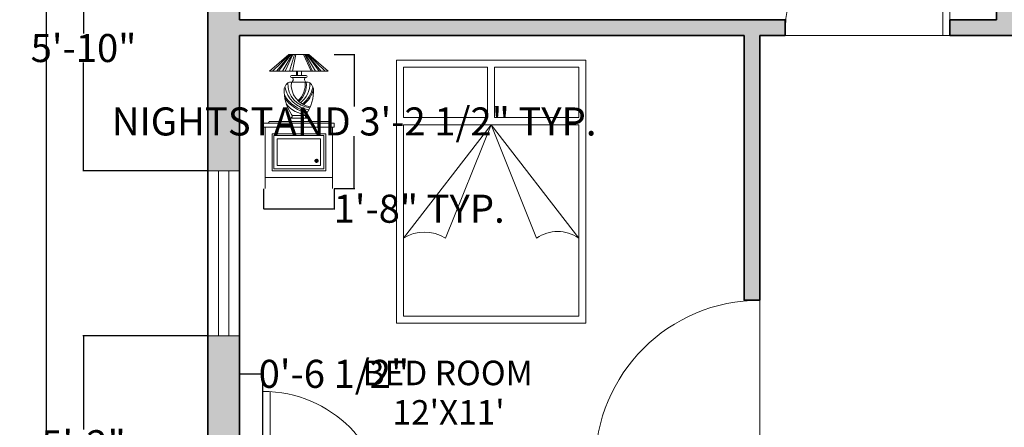
# Model space of a CAD drawing. Units: inches. Extents: x 638 to 1303, y 1 to 699.
# Tile 10 of 21: x 644 to 924, y 409 to 525. Entities that reach past the tile are written whole.
import ezdxf

# ---------------------------------------------------------------- set-up
doc = ezdxf.new("R2010")
doc.units = ezdxf.units.IN
doc.header["$MEASUREMENT"] = 0
for name, color, linetype, lineweight in [('A-ANNO-DIMS', 2, 'Continuous', 18), ('A-AREA-IDEN', 7, 'Continuous', 18), ('A-DOOR', 4, 'Continuous', 18), ('A-GLAZ', 4, 'Continuous', 18), ('A-WALL', 7, 'Continuous', 35), ('Furniture', 7, 'Continuous', 15)]:
    doc.layers.add(name, color=color, linetype=linetype, lineweight=lineweight)
doc.layers.add('A-WALL-PATT', color=143, linetype='Continuous', lineweight=13, true_color=0x7aafdf)
doc.styles.get("Standard").update_dxf_attribs({"font": 'arial.ttf'})
doc.dimstyles.get("Standard").update_dxf_attribs({"dimtxt": 8, "dimasz": 0.18, "dimexe": 0.18, "dimexo": 0.0625, "dimgap": 0.09, "dimtad": 0, "dimtih": 1, "dimtoh": 1, "dimdec": 4, "dimzin": 0, "dimdsep": 46, "dimlunit": 3, "dimtxsty": 'Standard', "dimcen": 0.09, "dimadec": 0, "dimazin": 0, "dimtfac": 1, "dimtdec": 4, "dimtofl": 0, "dimtmove": 0, "dimatfit": 3, "dimfxl": 1, "dimtolj": 1, "dimtzin": 0, "dimarcsym": 0})

# ---------------------------------------------------------------- blocks, each defined once
blk = doc.blocks.new('*D1')
at = {"layer": 'A-ANNO-DIMS', "color": 0, "lineweight": -2, "transparency": 16777216}
for p, q in [((697.18, 629.82), (650.92, 629.82)), ((651.1, 629.64), (651.1, 339.99)), ((651.1, 42), (651.1, 331.64)), ((697.18, 41.82), (650.92, 41.82))]:
    blk.add_line(p, q, dxfattribs=at)
at = {"layer": 'A-ANNO-DIMS', "color": 0, "transparency": 16777216}
for points in [[(651.07, 629.64), (651.13, 629.64), (651.1, 629.82)], [(651.07, 42), (651.13, 42), (651.1, 41.82)]]:
    blk.add_solid(points, dxfattribs=at)
at = {"layer": 'Defpoints', "color": 0, "transparency": 16777216}
for p in [(697.24, 629.82), (651.1, 41.82), (697.24, 41.82)]:
    blk.add_point(p, dxfattribs=at)
at = {"layer": 'A-ANNO-DIMS', "color": 0, "transparency": 16777216, "insert": (651.1, 335.82), "char_height": 8, "attachment_point": 5}
blk.add_mtext("\\A1;49'", dxfattribs=at)
blk = doc.blocks.new('DOOR-SWING-47')
for p, q in [((45, 0), (45, 46.96)), ((47, 0), (47, 47)), ((0, 0), (47, 0))]:
    blk.add_line(p, q)
blk.add_arc((47, 0), 47, 90, 180)
blk = doc.blocks.new('DOOR-SWING-35')
for p, q in [((33, 0), (33, 34.94)), ((35, 0), (35, 35)), ((0, 0), (35, 0))]:
    blk.add_line(p, q)
blk.add_arc((35, 0), 35, 90, 180)
blk = doc.blocks.new('WIN-47')
for p, q in [((47, 9), (0, 9)), ((0, 9), (0, 0)), ((47, 0), (47, 9)), ((0, 6), (47, 6)), ((0, 3), (47, 3)), ((0, 0), (47, 0))]:
    blk.add_line(p, q)
blk = doc.blocks.new('*X4')
at = {"color": 0}
for p, q in [((120.5, 200.05), (120.95, 200.5)), ((121, 199.5), (120.5, 200)), ((120.51, 199.89), (121.11, 200.49)), ((121.15, 199.52), (120.52, 200.15)), ((120.56, 199.76), (121.24, 200.44)), ((120.76, 199.56), (120.56, 199.76)), ((121.27, 199.58), (120.58, 200.27)), ((120.64, 199.66), (121.34, 200.36)), ((121.37, 199.66), (120.66, 200.37)), ((120.73, 199.58), (121.42, 200.27)), ((121.44, 199.76), (120.76, 200.44)), ((120.86, 199.52), (121.48, 200.14)), ((121.49, 199.89), (120.89, 200.49)), ((121.01, 199.5), (121.5, 199.99)), ((121.5, 200.06), (121.06, 200.5)), ((121.26, 199.57), (121.43, 199.74))]:
    blk.add_line(p, q, dxfattribs=at)
blk = doc.blocks.new('BEDSIDE-UNIT-WITH-LAMP')
for p, q in [((7.17, 38.27), (1.67, 33.48)), ((7.48, 38.27), (2.53, 33.48)), ((3.69, 33.48), (7.63, 38.27)), ((4.24, 33.48), (7.76, 38.27)), ((5.34, 33.48), (8.12, 38.27)), ((8.34, 38.27), (6.11, 33.48)), ((7.17, 38.27), (10.04, 38.27)), ((7.39, 33.48), (8.76, 38.27)), ((9.16, 38.27), (8.21, 33.48)), ((12.91, 38.27), (10.04, 38.27)), ((11.36, 38.27), (13.59, 33.48)), ((11.75, 38.27), (13.98, 33.48)), ((14.75, 33.48), (11.97, 38.27)), ((15.85, 33.48), (12.33, 38.27)), ((16.4, 33.48), (12.46, 38.27)), ((12.61, 38.27), (17.56, 33.48)), ((12.91, 38.27), (18.42, 33.48)), ((1.67, 33.48), (10.04, 33.48)), ((7.92, 32.29), (10.04, 32.29)), ((7.92, 31.69), (10.04, 31.69)), ((9.33, 32.29), (9.33, 33.48)), ((9.69, 32.29), (9.69, 33.48)), ((18.42, 33.48), (10.04, 33.48)), ((12.17, 32.29), (10.04, 32.29)), ((12.17, 31.69), (10.04, 31.69)), ((10.76, 32.29), (10.76, 33.48)), ((7.61, 30.38), (10.04, 30.38)), ((12.48, 30.38), (10.04, 30.38)), ((7.62, 20.09), (10.04, 20.09)), ((8.13, 20.83), (11.96, 20.83)), ((12.47, 20.09), (10.04, 20.09)), ((0, 18.66), (1.18, 18.66)), ((0, 18.66), (0, 17.54)), ((0, 17.54), (0.48, 17.54)), ((0.48, 17.54), (19.61, 17.54)), ((0.48, 17.54), (0.48, 0)), ((1.18, 18.66), (18.91, 18.66)), ((1.59, 19.13), (18.5, 19.13)), ((7.62, 19.13), (10.04, 19.13)), ((12.47, 19.13), (10.04, 19.13)), ((20.09, 18.66), (18.91, 18.66)), ((19.61, 17.54), (19.61, 0)), ((20.09, 17.54), (19.61, 17.54)), ((20.09, 18.66), (20.09, 17.54)), ((2.39, 15.63), (2.39, 5.1)), ((2.39, 15.63), (17.7, 15.63)), ((2.87, 15.15), (2.87, 5.58)), ((2.87, 15.15), (17.22, 15.15)), ((3.83, 14.19), (3.83, 6.54)), ((3.83, 14.19), (16.26, 14.19)), ((16.26, 14.19), (16.26, 6.54)), ((17.22, 15.15), (17.22, 5.58)), ((17.7, 15.63), (17.7, 5.1)), ((3.83, 6.54), (16.26, 6.54)), ((0.48, 3.19), (19.61, 3.19)), ((2.39, 5.1), (17.7, 5.1)), ((2.87, 5.58), (17.22, 5.58))]:
    blk.add_line(p, q)
blk.add_circle((15.11, 7.93), 0.478)
for centre, radius, start, end in [((7.95, 31.99), 0.301, 96.0644, 263.9356), ((7.75, 31.04), 0.677, 281.8983, 74.8511), ((12.34, 31.04), 0.677, 105.1489, 258.1017), ((12.14, 31.99), 0.301, 276.0644, 83.9356), ((17.45, 27.82), 11.6, 176.8022, 215.2924), ((9.63, 27.32), 3.94, 137.4597, 163.1575), ((14, 30.46), 8.06, 190.3097, 262.4706), ((7.61, 29.18), 1.2, 90, 137.4597), ((13.81, 29.96), 6.94, 178.6681, 265.1492), ((14.31, 29.63), 6.43, 173.3103, 261.113), ((5.78, 29.63), 6.07, 311.5876, 6.6897), ((5.78, 29.63), 6.43, 311.5876, 6.6897), ((6.28, 29.96), 6.94, 307.422, 1.3319), ((6.09, 30.46), 8.06, 307.8159, 349.6903), ((6.09, 30.46), 8.42, 308.8588, 345.4877), ((2.64, 27.82), 11.6, 324.7076, 3.1978), ((12.48, 29.18), 1.2, 42.5403, 90), ((10.46, 27.32), 3.94, 16.8425, 42.5403), ((14.79, 32.06), 10.42, 211.5602, 257.9287), ((14.79, 32.06), 10.78, 215.6196, 257.2465), ((12.31, 28.5), 7.31, 216.5807, 268.9053), ((7.65, 19.61), 0.479, 93.7182, 266.2818), ((7.53, 20.69), 0.609, 278.5359, 43.5342), ((12.56, 20.69), 0.609, 136.4658, 261.4641), ((12.44, 19.61), 0.479, 273.7182, 86.2818), ((1.05, 19.19), 0.546, 283.3604, 354.4124), ((19.04, 19.19), 0.546, 185.5876, 256.6396)]:
    blk.add_arc(centre, radius, start, end)
at = {"xscale": 0.956691, "yscale": 0.956691, "zscale": 0.956691}
blk.add_blockref('*X4', (-100.65, -183.4), dxfattribs=at)
blk = doc.blocks.new('*D34')
at = {"layer": 'A-ANNO-DIMS', "color": 0, "lineweight": -2, "transparency": 16777216}
for p, q in [((733.29, 514.93), (739.15, 514.93)), ((738.97, 514.75), (738.97, 500.03)), ((738.97, 476.84), (738.97, 491.57)), ((733.29, 476.66), (739.15, 476.66))]:
    blk.add_line(p, q, dxfattribs=at)
at = {"layer": 'A-ANNO-DIMS', "color": 0, "transparency": 16777216}
for points in [[(738.94, 514.75), (739, 514.75), (738.97, 514.93)], [(738.94, 476.84), (739, 476.84), (738.97, 476.66)]]:
    blk.add_solid(points, dxfattribs=at)
at = {"layer": 'Defpoints', "color": 0, "transparency": 16777216}
for p in [(733.23, 514.93), (738.97, 514.93), (733.23, 476.66)]:
    blk.add_point(p, dxfattribs=at)
at = {"layer": 'A-ANNO-DIMS', "color": 0, "transparency": 16777216, "insert": (738.97, 495.8), "char_height": 8, "attachment_point": 5}
blk.add_mtext('\\A1;NIGHTSTAND 3\'-2 1/2" TYP.', dxfattribs=at)
blk = doc.blocks.new('*D35')
at = {"layer": 'A-ANNO-DIMS', "color": 0, "lineweight": -2, "transparency": 16777216}
for p, q in [((713.14, 476.6), (713.14, 470.74)), ((733.23, 476.6), (733.23, 470.74)), ((713.32, 470.92), (733.05, 470.92)), ((733.23, 470.92), (733.41, 470.92))]:
    blk.add_line(p, q, dxfattribs=at)
at = {"layer": 'A-ANNO-DIMS', "color": 0, "transparency": 16777216}
for points in [[(713.32, 470.95), (713.32, 470.89), (713.14, 470.92)], [(733.05, 470.95), (733.05, 470.89), (733.23, 470.92)]]:
    blk.add_solid(points, dxfattribs=at)
at = {"layer": 'Defpoints', "color": 0, "transparency": 16777216}
for p in [(713.14, 476.66), (733.23, 476.66), (733.23, 470.92)]:
    blk.add_point(p, dxfattribs=at)
at = {"layer": 'A-ANNO-DIMS', "color": 0, "transparency": 16777216, "insert": (757.51, 470.92), "char_height": 8, "attachment_point": 5}
blk.add_mtext('\\A1;1\'-8" TYP.', dxfattribs=at)
blk = doc.blocks.new('*D58')
at = {"layer": 'A-ANNO-DIMS', "color": 0, "lineweight": -2, "transparency": 16777216}
for p, q in [((697.18, 434.7), (661.56, 434.7)), ((661.74, 434.52), (661.74, 407.92)), ((661.74, 372.97), (661.74, 399.57)), ((697.18, 372.79), (661.56, 372.79))]:
    blk.add_line(p, q, dxfattribs=at)
at = {"layer": 'A-ANNO-DIMS', "color": 0, "transparency": 16777216}
for points in [[(661.71, 434.52), (661.77, 434.52), (661.74, 434.7)], [(661.71, 372.97), (661.77, 372.97), (661.74, 372.79)]]:
    blk.add_solid(points, dxfattribs=at)
at = {"layer": 'Defpoints', "color": 0, "transparency": 16777216}
for p in [(661.74, 434.7), (697.24, 434.7), (697.24, 372.79)]:
    blk.add_point(p, dxfattribs=at)
at = {"layer": 'A-ANNO-DIMS', "color": 0, "transparency": 16777216, "insert": (661.74, 403.75), "char_height": 8, "attachment_point": 5}
blk.add_mtext('\\A1;5\'-2"', dxfattribs=at)
blk = doc.blocks.new('*D59')
at = {"layer": 'A-ANNO-DIMS', "color": 0, "lineweight": -2, "transparency": 16777216}
for p, q in [((697.18, 551.77), (661.56, 551.77)), ((661.74, 551.59), (661.74, 520.91)), ((661.74, 481.88), (661.74, 512.57)), ((697.18, 481.7), (661.56, 481.7))]:
    blk.add_line(p, q, dxfattribs=at)
at = {"layer": 'A-ANNO-DIMS', "color": 0, "transparency": 16777216}
for points in [[(661.71, 551.59), (661.77, 551.59), (661.74, 551.77)], [(661.71, 481.88), (661.77, 481.88), (661.74, 481.7)]]:
    blk.add_solid(points, dxfattribs=at)
at = {"layer": 'Defpoints', "color": 0, "transparency": 16777216}
for p in [(661.74, 551.77), (697.24, 551.77), (697.24, 481.7)]:
    blk.add_point(p, dxfattribs=at)
at = {"layer": 'A-ANNO-DIMS', "color": 0, "transparency": 16777216, "insert": (661.74, 516.74), "char_height": 8, "attachment_point": 5}
blk.add_mtext('\\A1;5\'-10"', dxfattribs=at)
blk = doc.blocks.new('*D70')
at = {"layer": 'A-ANNO-DIMS', "color": 0, "lineweight": -2, "transparency": 16777216}
for p, q in [((706.24, 388.38), (706.24, 424)), ((706.42, 423.82), (712.77, 423.82)), ((712.95, 388.38), (712.95, 424)), ((712.95, 423.82), (713.13, 423.82))]:
    blk.add_line(p, q, dxfattribs=at)
at = {"layer": 'A-ANNO-DIMS', "color": 0, "transparency": 16777216}
for points in [[(706.42, 423.85), (706.42, 423.79), (706.24, 423.82)], [(712.77, 423.85), (712.77, 423.79), (712.95, 423.82)]]:
    blk.add_solid(points, dxfattribs=at)
at = {"layer": 'Defpoints', "color": 0, "transparency": 16777216}
for p in [(712.95, 423.82), (706.24, 388.32), (712.95, 388.32)]:
    blk.add_point(p, dxfattribs=at)
at = {"layer": 'A-ANNO-DIMS', "color": 0, "transparency": 16777216, "insert": (733.18, 423.82), "char_height": 8, "attachment_point": 5}
blk.add_mtext('\\A1;0\'-6 1/2"', dxfattribs=at)

msp = doc.modelspace()

# ---------------------------------------------------------------- hatches: boundary and pattern name
at = {"layer": 'A-WALL-PATT'}
h = msp.add_hatch(color=256, dxfattribs=at)
h.dxf.hatch_style = 1
h.paths.add_polyline_path([(973.34524, 629.81895), (793.35541, 629.81895), (793.35541, 620.81895), (850.23798, 620.81895), (922.23798, 620.81895), (922.23798, 524.81895), (908.94335, 524.81895), (908.94335, 520.31895), (926.73798, 520.31895), (926.73798, 544.31895), (979.3571, 544.31895), (979.3571, 548.81895), (926.73798, 548.81895), (926.73798, 620.81895), (973.34524, 620.81895)])
h.paths.add_polyline_path([(758.35541, 629.81895), (697.23798, 629.81895), (697.23798, 586.77451), (706.23798, 586.77451), (706.23798, 620.81895), (758.35541, 620.81895)])
h.paths.add_polyline_path([(1075.85281, 629.81895), (1003.34524, 629.81895), (1003.34524, 620.81895), (1046.73798, 620.81895), (1046.73798, 560.81895), (1046.73798, 548.81895), (1026.3571, 548.81895), (1026.3571, 544.31895), (1046.73798, 544.31895), (1046.73798, 486.87457), (1051.23798, 486.87457), (1051.23798, 556.31895), (1162.89753, 556.31895), (1162.89753, 560.81895), (1051.23798, 560.81895), (1051.23798, 620.81895), (1075.85281, 620.81895)])
h.paths.add_polyline_path([(1228.23798, 629.81895), (1105.85281, 629.81895), (1105.85281, 620.81895), (1219.23798, 620.81895), (1219.23798, 560.81895), (1197.89753, 560.81895), (1197.89753, 556.31895), (1219.23798, 556.31895), (1219.23798, 498.80084), (1228.23798, 498.80084)])
h.paths.add_polyline_path([(1051.23798, 439.87457), (1046.73798, 439.87457), (1046.73798, 407.81895), (1219.23798, 407.81895), (1219.23798, 381.66175), (1228.23798, 381.66175), (1228.23798, 451.80084), (1219.23798, 451.80084), (1219.23798, 412.31895), (1051.23798, 412.31895)])
h.paths.add_polyline_path([(1228.23798, 346.66175), (1219.23798, 346.66175), (1219.23798, 335.81895), (1046.73798, 335.81895), (1046.73798, 273.56895), (1051.23798, 273.56895), (1051.23798, 331.31895), (1219.23798, 331.31895), (1219.23798, 308.99654), (1228.23798, 308.99654)])
h.paths.add_polyline_path([(1228.23798, 261.99654), (1219.23798, 261.99654), (1219.23798, 211.31895), (1051.23798, 211.31895), (1051.23798, 226.56895), (1046.73798, 226.56895), (1046.73798, 211.31895), (983.84714, 211.31895), (983.84714, 206.81895), (1219.23798, 206.81895), (1219.23798, 166.83987), (1228.23798, 166.83987)])
h.paths.add_polyline_path([(1228.23798, 119.83987), (1219.23798, 119.83987), (1219.23798, 50.81895), (1197.89277, 50.81895), (1197.89277, 41.81895), (1228.23798, 41.81895)])
h.paths.add_polyline_path([(1162.89277, 50.81895), (1069.02949, 50.81895), (1069.02949, 41.81895), (1162.89277, 41.81895)])
h.paths.add_polyline_path([(1010.02949, 50.81895), (941.89631, 50.81895), (917.77455, 50.81895), (917.77455, 41.81895), (941.89631, 41.81895), (1010.02949, 41.81895)])
h.paths.add_polyline_path([(882.77455, 50.81895), (854.73798, 50.81895), (854.73798, 145.50379), (850.23798, 145.50379), (850.23798, 50.81895), (793.49755, 50.81895), (793.49755, 41.81895), (882.77455, 41.81895)])
h.paths.add_polyline_path([(746.49755, 50.81895), (706.23798, 50.81895), (706.23798, 96.57416), (697.23798, 96.57416), (697.23798, 41.81895), (746.49755, 41.81895)])
h.paths.add_polyline_path([(706.23798, 206.81895), (714.01165, 206.81895), (714.01165, 211.31895), (706.23798, 211.31895), (706.23798, 251.21966), (697.23798, 251.21966), (697.23798, 143.57416), (706.23798, 143.57416)])
h.paths.add_polyline_path([(923.84714, 211.31895), (854.73798, 211.31895), (854.73798, 397.8313), (850.23798, 397.8313), (850.23798, 388.31895), (747.9539, 388.31895), (747.9539, 383.81895), (850.23798, 383.81895), (850.23798, 311.81895), (706.23798, 311.81895), (706.23798, 342.78787), (697.23798, 342.78787), (697.23798, 281.21966), (706.23798, 281.21966), (706.23798, 307.31895), (850.23798, 307.31895), (850.23798, 211.31895), (749.01165, 211.31895), (749.01165, 206.81895), (850.23798, 206.81895), (850.23798, 192.50379), (854.73798, 192.50379), (854.73798, 206.81895), (923.84714, 206.81895)])
h.paths.add_polyline_path([(706.23798, 434.70471), (697.23798, 434.70471), (697.23798, 372.78787), (706.23798, 372.78787), (706.23798, 383.81895), (712.9539, 383.81895), (712.9539, 388.31895), (706.23798, 388.31895)])
h.paths.add_polyline_path([(706.23798, 520.31895), (850.23798, 520.31895), (850.23798, 444.8313), (854.73798, 444.8313), (854.73798, 520.31895), (861.94335, 520.31895), (861.94335, 524.81895), (706.23798, 524.81895), (706.23798, 551.77451), (697.23798, 551.77451), (697.23798, 481.70471), (706.23798, 481.70471)])

# ---------------------------------------------------------------- linework, layer by layer
at = {"layer": 'A-DOOR'}
msp.add_line((854.73798, 444.8313), (854.73798, 397.8313), dxfattribs=at)
msp.add_arc((854.73798, 397.8313), 47, 90, 180, dxfattribs=at)
at = {"layer": 'A-WALL'}
for p, q in [((697.23798, 41.81895), (697.23798, 629.81895)), ((706.23798, 524.81895), (706.23798, 620.81895)), ((922.23798, 524.81895), (922.23798, 620.81895)), ((861.94335, 524.81895), (706.23798, 524.81895)), ((861.94335, 524.81895), (861.94335, 520.31895)), ((922.23798, 524.81895), (908.94335, 524.81895)), ((908.94335, 524.81895), (908.94335, 520.31895)), ((706.23798, 388.31895), (706.23798, 520.31895)), ((850.23798, 520.31895), (706.23798, 520.31895)), ((850.23798, 444.8313), (850.23798, 520.31895)), ((861.94335, 520.31895), (854.73798, 520.31895)), ((854.73798, 444.8313), (854.73798, 520.31895)), ((926.73798, 520.31895), (908.94335, 520.31895)), ((850.23798, 444.8313), (854.73798, 444.8313))]:
    msp.add_line(p, q, dxfattribs=at)
at = {"layer": 'Furniture'}
for p, q in [((751.03478, 513.26636), (805.03478, 513.26636)), ((751.03478, 438.26636), (751.03478, 513.26636)), ((805.03478, 513.26636), (805.03478, 438.26636)), ((753.03478, 511.26636), (777.03478, 511.26636)), ((753.03478, 496.88333), (753.03478, 511.26636)), ((777.03478, 496.88333), (777.03478, 511.26636)), ((779.03478, 496.88333), (779.03478, 511.26636)), ((779.03478, 511.26636), (803.03478, 511.26636)), ((803.03478, 511.26636), (803.03478, 496.88333)), ((753.03478, 496.88333), (777.03478, 496.88333)), ((753.03478, 440.26636), (753.03478, 494.88333)), ((753.03478, 494.88333), (803.03478, 494.88333)), ((778.03478, 494.88333), (753.03478, 462.56111)), ((765.03478, 462.56111), (778.03478, 494.88333)), ((778.03478, 494.88333), (803.03478, 462.56111)), ((791.03478, 462.56111), (778.03478, 494.88333)), ((779.03478, 496.88333), (803.03478, 496.88333)), ((803.03478, 494.88333), (803.03478, 440.26636)), ((803.03478, 440.26636), (753.03478, 440.26636)), ((805.03478, 438.26636), (751.03478, 438.26636))]:
    msp.add_line(p, q, dxfattribs=at)
for centre, radius, start, end in [((759.03478, 452.65347), 11.5828, 58.8011862, 121.1988138), ((797.03478, 453.7632), 10.6491, 55.7067931, 124.2932069)]:
    msp.add_arc(centre, radius, start, end, dxfattribs=at)

# ---------------------------------------------------------------- block references
at = {"layer": 'A-DOOR'}
msp.add_blockref('DOOR-SWING-47', (861.943, 520.319), dxfattribs=at)
at = {"layer": 'A-DOOR', "extrusion": (0, 0, -1), "zscale": -1}
msp.add_blockref('DOOR-SWING-35', (-747.95343, 383.819), dxfattribs=at)
at = {"layer": 'A-GLAZ', "rotation": 270}
msp.add_blockref('WIN-47', (697.23803, 481.70426), dxfattribs=at)
at = {"layer": 'Furniture'}
msp.add_blockref('BEDSIDE-UNIT-WITH-LAMP', (713.13976, 476.66272), dxfattribs=at)

# ---------------------------------------------------------------- texts
at = {"layer": 'A-AREA-IDEN'}
for s, p in [('BED ROOM ', (741.35813, 420.57544)), ("    12'X11'", (741.35813, 409.33056))]:
    msp.add_text(s, height=7, dxfattribs=at).set_placement(p)

# ---------------------------------------------------------------- dimensions: what is measured, and where the dimension line sits
at = {"layer": 'A-ANNO-DIMS'}
for base, p1, p2, override, picture, middle in [((651.10111, 41.81895), (697.23798, 629.81895), (697.23798, 41.81895), {"dimclrd": 0, "dimclre": 0, "dimclrt": 0}, '*D1', (651.10111, 335.81895)), ((661.73798, 551.77451), (697.23798, 481.70471), (697.23798, 551.77451), {"dimdec": 1, "dimlfac": 1, "dimrnd": 0, "dimzin": 1, "dimdsep": 46, "dimlunit": 4, "dimfrac": 2}, '*D59', (661.73798, 516.73961)), ((661.73798, 434.70471), (697.23798, 372.78787), (697.23798, 434.70471), {"dimdec": 1, "dimlfac": 1, "dimrnd": 0, "dimzin": 1, "dimdsep": 46, "dimlunit": 4, "dimfrac": 2}, '*D58', (661.73798, 403.74629))]:
    dim = msp.add_linear_dim(base=base, p1=p1, p2=p2, angle=90, dimstyle='Standard', override=override, dxfattribs=at)
    dim.commit()
    dim.dimension.update_dxf_attribs({"geometry": picture, "text_midpoint": middle})
dim = msp.add_linear_dim(base=(738.97004, 514.93085), p1=(733.22989, 476.66321), p2=(733.22989, 514.93085), angle=90, text='NIGHTSTAND <> TYP.', dimstyle='Standard', override={"dimdec": 1, "dimlfac": 1, "dimrnd": 0, "dimzin": 1, "dimdsep": 46, "dimlunit": 4, "dimfrac": 2}, dxfattribs=at)
dim.commit()
dim.dimension.update_dxf_attribs({"geometry": '*D34', "text_midpoint": (738.97004, 495.79703)})
dim = msp.add_linear_dim(base=(733.22989, 470.92307), p1=(713.13938, 476.66321), p2=(733.22989, 476.66321), text='<> TYP.', dimstyle='Standard', override={"dimdec": 1, "dimlfac": 1, "dimrnd": 0, "dimzin": 1, "dimdsep": 46, "dimlunit": 4, "dimfrac": 2}, dxfattribs=at)
dim.commit()
dim.dimension.update_dxf_attribs({"geometry": '*D35', "text_midpoint": (757.50535, 470.92307)})
dim = msp.add_linear_dim(base=(712.9539, 423.81895), p1=(706.23798, 388.31895), p2=(712.9539, 388.31895), dimstyle='Standard', override={"dimdec": 1, "dimlfac": 1, "dimrnd": 0, "dimzin": 1, "dimdsep": 46, "dimlunit": 4, "dimfrac": 2}, dxfattribs=at)
dim.commit()
dim.dimension.update_dxf_attribs({"geometry": '*D70', "text_midpoint": (733.17752, 423.81895)})

doc.saveas('drawing.dxf')
